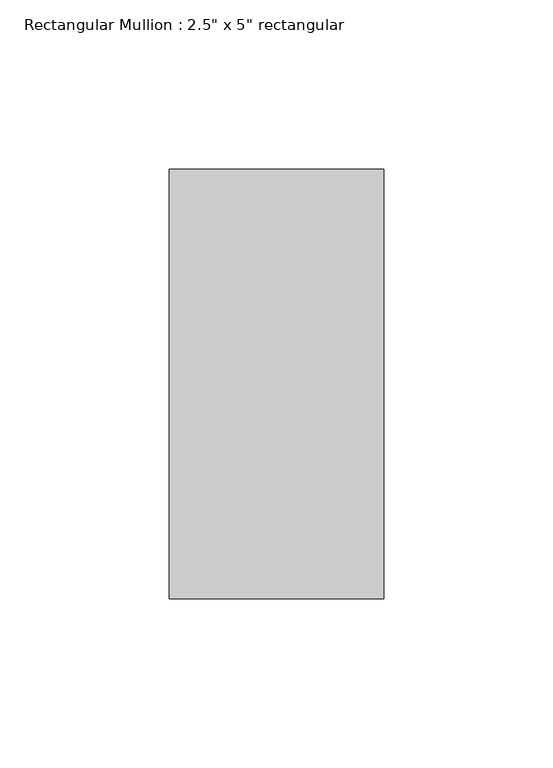
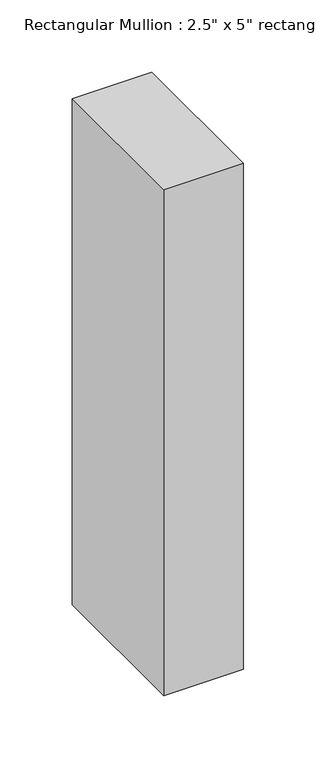
"""IFC4 building model written with IfcOpenShell, lengths in millimetres: member geometry."""

from ifc_helpers import new_model, si_unit, frame, origin, place, context, project, spatial, polyline, outline, extrude, source, transform, mapped, element, save


def member_39486dda(model_context):
    return source(origin(), model_context, "Body", "SweptSolid", [
        extrude(outline(polyline([(0.0, 63.5), (0.0, -63.5), (-63.5, -63.5), (-63.5, 63.5), (0.0, 63.5)])), frame((0.0, 0.0, -427.5666667), z_axis=(0.0, 0.0, 1.0), x_axis=(1.0, 0.0, 0.0)), (0.0, 0.0, 1.0), 427.5666667),
    ])


if __name__ == "__main__":
    model = new_model("IFC4")
    model_context = context("Model", 3, world=origin())
    ifc_project = project(units=[si_unit("LENGTHUNIT", "METRE", prefix="MILLI")], contexts=[model_context])
    site = spatial("IfcSite", under=ifc_project)
    building = spatial("IfcBuilding", under=site)
    placement = place(None, origin())
    member_shape = member_39486dda(model_context)
    element("IfcMember", 1, ObjectType="Rectangular Mullion : 2.5\" x 5\" rectangular", at=placement, inside=building, context=model_context, shape_type="MappedRepresentation", body=[
        mapped(member_shape, transform((0.0, 0.0, 0.0), x_axis=(1.0, 0.0, 0.0), y_axis=(0.0, 1.0, 0.0), z_axis=(0.0, 0.0, 1.0))),
    ])
    save(model, "model.ifc")

# Revit data of these elements
# Type "Rectangular Mullion : 2.5\" x 5\" rectangular"
#   built-in parameter 1007304 = 0.416667 (stored number, unit not read)
#   built-in parameter 1007301 = 0.104167 (stored number, unit not read)
#   built-in parameter 1007300 = 0.104167 (stored number, unit not read)
# Element 1 (IfcMember, "Rectangular Mullion : 2.5\" x 5\" rectangular")
#   Materials on its faces: "Aluminum"
# Materials
#   "Aluminum": class "Metal", colour RGB 247 247 247, transparency 0, Description = "Aluminum 6061", Cost = 0
